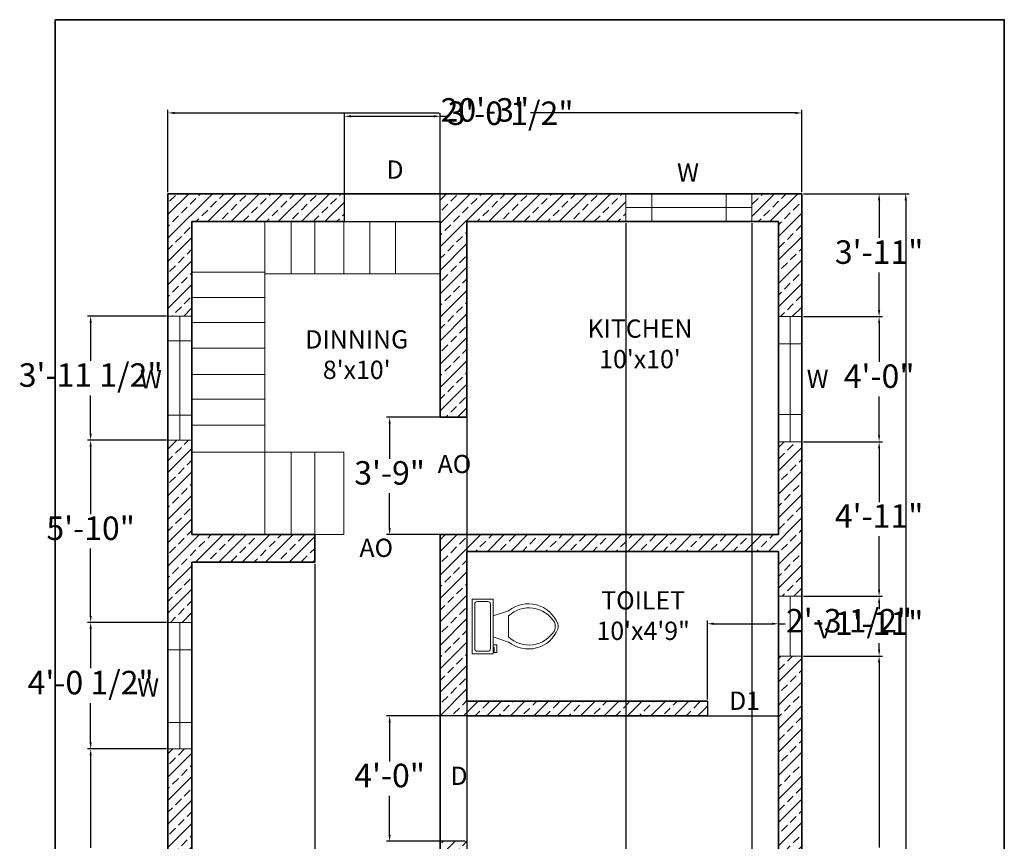
# Model space of a CAD drawing. Units: inches. Extents: x 3686 to 4476, y 4404 to 5066.
# Tile 2 of 2: x 3686 to 4064, y 4751 to 5066. Entities that reach past the tile are written whole.
import ezdxf

# ---------------------------------------------------------------- set-up
doc = ezdxf.new("R2010")
doc.units = ezdxf.units.IN
for name, color, linetype, lineweight in [('A-ANNO-DIMS', 3, 'Continuous', 18), ('A-ANNO-TEXT', 7, 'Continuous', 18), ('A-ANNO-TTLB', 7, 'Continuous', 35), ('A-AREA-IDEN', 7, 'Continuous', 25), ('A-DOOR', 3, 'Continuous', 25), ('A-FLOR-FIXT', 9, 'Continuous', 18), ('A-FLOR-STRS', 7, 'Continuous', 18), ('A-GLAZ', 4, 'Continuous', 18), ('A-WALL', 7, 'Continuous', 35), ('A-WALL-PATT', 8, 'Continuous', 13)]:
    doc.layers.add(name, color=color, linetype=linetype, lineweight=lineweight)
doc.styles.get("Standard").update_dxf_attribs({"font": 'arial.ttf'})
doc.dimstyles.new('ISO-25', dxfattribs={"dimtxt": 9, "dimasz": 2.5, "dimexe": 1.25, "dimexo": 0.625, "dimgap": 2, "dimtad": 0, "dimtih": 1, "dimtoh": 1, "dimdec": 1, "dimlunit": 4, "dimtxsty": 'Standard', "dimcen": 2.5, "dimadec": 0, "dimazin": 0, "dimtfac": 0.5, "dimtdec": 1, "dimtmove": 0, "dimatfit": 3, "dimfxl": 1, "dimarcsym": 0})

# ---------------------------------------------------------------- blocks, each defined once
blk = doc.blocks.new('*D1')
at = {"layer": 'A-ANNO-DIMS', "color": 0, "lineweight": -2, "transparency": 16777216}
for p, q in [((3743.02, 4999.94), (3743.02, 5031.48)), ((3745.52, 5030.23), (3846.98, 5030.23)), ((3983.52, 5030.23), (3882.05, 5030.23)), ((3986.02, 4999.94), (3986.02, 5031.48))]:
    blk.add_line(p, q, dxfattribs=at)
at = {"layer": 'A-ANNO-DIMS', "color": 0, "transparency": 16777216}
for points in [[(3745.52, 5030.65), (3745.52, 5029.82), (3743.02, 5030.23)], [(3983.52, 5030.65), (3983.52, 5029.82), (3986.02, 5030.23)]]:
    blk.add_solid(points, dxfattribs=at)
at = {"layer": 'Defpoints', "color": 0, "transparency": 16777216}
for p in [(3986.02, 5030.23), (3743.02, 4999.31), (3986.02, 4999.31)]:
    blk.add_point(p, dxfattribs=at)
at = {"layer": 'A-ANNO-DIMS', "color": 0, "transparency": 16777216, "insert": (3864.52, 5030.23), "char_height": 9, "attachment_point": 5}
blk.add_mtext('20\'-3"', dxfattribs=at)
blk = doc.blocks.new('*D2')
at = {"layer": 'A-ANNO-DIMS', "color": 0, "lineweight": -2, "transparency": 16777216}
for p, q in [((3986.64, 4999.31), (4027.13, 4999.31)), ((4025.88, 4996.81), (4025.88, 4729.91)), ((4025.88, 4449.81), (4025.88, 4716.72)), ((3986.64, 4447.31), (4027.13, 4447.31))]:
    blk.add_line(p, q, dxfattribs=at)
at = {"layer": 'A-ANNO-DIMS', "color": 0, "transparency": 16777216}
for points in [[(4025.46, 4996.81), (4026.3, 4996.81), (4025.88, 4999.31)], [(4025.46, 4449.81), (4026.3, 4449.81), (4025.88, 4447.31)]]:
    blk.add_solid(points, dxfattribs=at)
at = {"layer": 'Defpoints', "color": 0, "transparency": 16777216}
for p in [(3986.02, 4999.31), (3986.02, 4447.31), (4025.88, 4447.31)]:
    blk.add_point(p, dxfattribs=at)
at = {"layer": 'A-ANNO-DIMS', "color": 0, "transparency": 16777216, "insert": (4025.88, 4723.31), "char_height": 9, "attachment_point": 5}
blk.add_mtext("46'", dxfattribs=at)
blk = doc.blocks.new('*U6')
for p, q in [((9.5, -6), (9.5, -2)), ((-10, -8.5), (-8, -8.5)), ((-10, -9.5), (-10, -8.5)), ((-7, -9.5), (-10, -9.5)), ((-8, -8.5), (-8, -8)), ((-7, -8), (-7, -9.5)), ((-4, -8), (-6, -14)), ((4, -8), (6, -14)), ((4, -14), (-4, -14))]:
    blk.add_line(p, q)
blk.add_lwpolyline([(10.5, -8), (10.5, 0), (-10.5, 0), (-10.5, -8)], close=True)
for points in [[(-9.5, -2), (-9.5, -6)], [(8.5, -1), (-8.5, -1)], [(-8.5, -7), (8.5, -7)]]:
    blk.add_lwpolyline(points)
for centre, radius, start, end in [((-8.62, -1.88), 0.884, 81.8699, 188.1301), ((8.62, -1.88), 0.884, 351.8699, 98.1301), ((-8.62, -6.12), 0.884, 171.8699, 278.1301), ((8.62, -6.12), 0.884, 261.8699, 8.1301), ((3.52, -21.58), 12.17, 141.4691, 247.9714), ((4.2, -21.82), 11.33, 136.3677, 238.9468), ((-3.52, -21.58), 12.17, 292.0284, 38.5307), ((-4.2, -21.82), 11.33, 301.053, 43.6321), ((0, -27.88), 4, 245.7318, 294.2682), ((0, -29), 4, 254.8605, 285.1395)]:
    blk.add_arc(centre, radius, start, end)
blk = doc.blocks.new('*D13')
at = {"layer": 'A-ANNO-DIMS', "color": 0, "lineweight": -2, "transparency": 16777216}
for p, q in [((3810.64, 4989.22), (3810.64, 5030.21)), ((3813.14, 5028.96), (3844.89, 5028.96)), ((3847.39, 4989.22), (3847.39, 5030.21)), ((3847.39, 5028.96), (3849.89, 5028.96))]:
    blk.add_line(p, q, dxfattribs=at)
at = {"layer": 'A-ANNO-DIMS', "color": 0, "transparency": 16777216}
for points in [[(3813.14, 5029.38), (3813.14, 5028.55), (3810.64, 5028.96)], [(3844.89, 5029.38), (3844.89, 5028.55), (3847.39, 5028.96)]]:
    blk.add_solid(points, dxfattribs=at)
at = {"layer": 'Defpoints', "color": 0, "transparency": 16777216}
for p in [(3847.39, 5028.96), (3810.64, 4988.59), (3847.39, 4988.59)]:
    blk.add_point(p, dxfattribs=at)
at = {"layer": 'A-ANNO-DIMS', "color": 0, "transparency": 16777216, "insert": (3874.33, 5028.96), "char_height": 9, "attachment_point": 5}
blk.add_mtext('3\'-0 1/2"', dxfattribs=at)
blk = doc.blocks.new('*D14')
at = {"layer": 'A-ANNO-DIMS', "color": 0, "lineweight": -2, "transparency": 16777216}
for p, q in [((3857.64, 4987.97), (3857.64, 4416.41)), ((3918.61, 4987.97), (3918.61, 4416.41)), ((3860.14, 4417.66), (3874.16, 4417.66)), ((3916.11, 4417.66), (3902.09, 4417.66))]:
    blk.add_line(p, q, dxfattribs=at)
at = {"layer": 'A-ANNO-DIMS', "color": 0, "transparency": 16777216}
for points in [[(3860.14, 4418.08), (3860.14, 4417.25), (3857.64, 4417.66)], [(3916.11, 4418.08), (3916.11, 4417.25), (3918.61, 4417.66)]]:
    blk.add_solid(points, dxfattribs=at)
at = {"layer": 'Defpoints', "color": 0, "transparency": 16777216}
for p in [(3857.64, 4988.59), (3918.61, 4988.59), (3918.61, 4417.66)]:
    blk.add_point(p, dxfattribs=at)
at = {"layer": 'A-ANNO-DIMS', "color": 0, "transparency": 16777216, "insert": (3888.13, 4417.66), "char_height": 9, "attachment_point": 5}
blk.add_mtext('5\'-1"', dxfattribs=at)
blk = doc.blocks.new('*D15')
at = {"layer": 'A-ANNO-DIMS', "color": 0, "lineweight": -2, "transparency": 16777216}
for p, q in [((3918.61, 4987.97), (3918.61, 4416.41)), ((3966.81, 4987.97), (3966.81, 4416.41)), ((3921.11, 4417.66), (3928.57, 4417.66)), ((3964.31, 4417.66), (3956.85, 4417.66))]:
    blk.add_line(p, q, dxfattribs=at)
at = {"layer": 'A-ANNO-DIMS', "color": 0, "transparency": 16777216}
for points in [[(3921.11, 4418.08), (3921.11, 4417.25), (3918.61, 4417.66)], [(3964.31, 4418.08), (3964.31, 4417.25), (3966.81, 4417.66)]]:
    blk.add_solid(points, dxfattribs=at)
at = {"layer": 'Defpoints', "color": 0, "transparency": 16777216}
for p in [(3918.61, 4988.59), (3966.81, 4988.59), (3966.81, 4417.66)]:
    blk.add_point(p, dxfattribs=at)
at = {"layer": 'A-ANNO-DIMS', "color": 0, "transparency": 16777216, "insert": (3942.71, 4417.66), "char_height": 9, "attachment_point": 5}
blk.add_mtext('4\'-0"', dxfattribs=at)
blk = doc.blocks.new('*D16')
at = {"layer": 'A-ANNO-DIMS', "color": 0, "lineweight": -2, "transparency": 16777216}
for p, q in [((3986.64, 4999.31), (4016.92, 4999.31)), ((4015.67, 4996.81), (4015.67, 4982.36)), ((4015.67, 4954.71), (4015.67, 4969.16)), ((3986.64, 4952.21), (4016.92, 4952.21))]:
    blk.add_line(p, q, dxfattribs=at)
at = {"layer": 'A-ANNO-DIMS', "color": 0, "transparency": 16777216}
for points in [[(4015.25, 4996.81), (4016.08, 4996.81), (4015.67, 4999.31)], [(4015.25, 4954.71), (4016.08, 4954.71), (4015.67, 4952.21)]]:
    blk.add_solid(points, dxfattribs=at)
at = {"layer": 'Defpoints', "color": 0, "transparency": 16777216}
for p in [(3986.02, 4999.31), (3986.02, 4952.21), (4015.67, 4952.21)]:
    blk.add_point(p, dxfattribs=at)
at = {"layer": 'A-ANNO-DIMS', "color": 0, "transparency": 16777216, "insert": (4015.67, 4975.76), "char_height": 9, "attachment_point": 5}
blk.add_mtext('3\'-11"', dxfattribs=at)
blk = doc.blocks.new('*D17')
at = {"layer": 'A-ANNO-DIMS', "color": 0, "lineweight": -2, "transparency": 16777216}
for p, q in [((3986.64, 4952.21), (4016.92, 4952.21)), ((4015.67, 4949.71), (4015.67, 4934.82)), ((4015.67, 4906.73), (4015.67, 4921.63)), ((3986.64, 4904.23), (4016.92, 4904.23))]:
    blk.add_line(p, q, dxfattribs=at)
at = {"layer": 'A-ANNO-DIMS', "color": 0, "transparency": 16777216}
for points in [[(4015.25, 4949.71), (4016.08, 4949.71), (4015.67, 4952.21)], [(4015.25, 4906.73), (4016.08, 4906.73), (4015.67, 4904.23)]]:
    blk.add_solid(points, dxfattribs=at)
at = {"layer": 'Defpoints', "color": 0, "transparency": 16777216}
for p in [(3986.02, 4952.21), (3986.02, 4904.23), (4015.67, 4904.23)]:
    blk.add_point(p, dxfattribs=at)
at = {"layer": 'A-ANNO-DIMS', "color": 0, "transparency": 16777216, "insert": (4015.67, 4928.22), "char_height": 9, "attachment_point": 5}
blk.add_mtext('4\'-0"', dxfattribs=at)
blk = doc.blocks.new('*D18')
at = {"layer": 'A-ANNO-DIMS', "color": 0, "lineweight": -2, "transparency": 16777216}
for p, q in [((3986.64, 4904.23), (4016.92, 4904.23)), ((4015.67, 4901.73), (4015.67, 4881.17)), ((4015.67, 4847.58), (4015.67, 4868.14)), ((3986.64, 4845.08), (4016.92, 4845.08))]:
    blk.add_line(p, q, dxfattribs=at)
at = {"layer": 'A-ANNO-DIMS', "color": 0, "transparency": 16777216}
for points in [[(4015.25, 4901.73), (4016.08, 4901.73), (4015.67, 4904.23)], [(4015.25, 4847.58), (4016.08, 4847.58), (4015.67, 4845.08)]]:
    blk.add_solid(points, dxfattribs=at)
at = {"layer": 'Defpoints', "color": 0, "transparency": 16777216}
for p in [(3986.02, 4904.23), (3986.02, 4845.08), (4015.67, 4845.08)]:
    blk.add_point(p, dxfattribs=at)
at = {"layer": 'A-ANNO-DIMS', "color": 0, "transparency": 16777216, "insert": (4015.67, 4874.65), "char_height": 9, "attachment_point": 5}
blk.add_mtext('4\'-11"', dxfattribs=at)
blk = doc.blocks.new('*D19')
at = {"layer": 'A-ANNO-DIMS', "color": 0, "lineweight": -2, "transparency": 16777216}
for p, q in [((3986.64, 4845.08), (4016.92, 4845.08)), ((4015.67, 4842.58), (4015.67, 4840.11)), ((4015.67, 4824.62), (4015.67, 4827.08)), ((3986.64, 4822.12), (4016.92, 4822.12))]:
    blk.add_line(p, q, dxfattribs=at)
at = {"layer": 'A-ANNO-DIMS', "color": 0, "transparency": 16777216}
for points in [[(4015.25, 4842.58), (4016.08, 4842.58), (4015.67, 4845.08)], [(4015.25, 4824.62), (4016.08, 4824.62), (4015.67, 4822.12)]]:
    blk.add_solid(points, dxfattribs=at)
at = {"layer": 'Defpoints', "color": 0, "transparency": 16777216}
for p in [(3986.02, 4845.08), (3986.02, 4822.12), (4015.67, 4822.12)]:
    blk.add_point(p, dxfattribs=at)
at = {"layer": 'A-ANNO-DIMS', "color": 0, "transparency": 16777216, "insert": (4015.67, 4833.6), "char_height": 9, "attachment_point": 5}
blk.add_mtext('1\'-11"', dxfattribs=at)
blk = doc.blocks.new('*D20')
at = {"layer": 'A-ANNO-DIMS', "color": 0, "lineweight": -2, "transparency": 16777216}
for p, q in [((3986.64, 4822.12), (4016.92, 4822.12)), ((4015.67, 4819.62), (4015.67, 4748.74)), ((4015.67, 4664.68), (4015.67, 4735.55)), ((3986.64, 4662.18), (4016.92, 4662.18))]:
    blk.add_line(p, q, dxfattribs=at)
at = {"layer": 'A-ANNO-DIMS', "color": 0, "transparency": 16777216}
for points in [[(4015.25, 4819.62), (4016.08, 4819.62), (4015.67, 4822.12)], [(4015.25, 4664.68), (4016.08, 4664.68), (4015.67, 4662.18)]]:
    blk.add_solid(points, dxfattribs=at)
at = {"layer": 'Defpoints', "color": 0, "transparency": 16777216}
for p in [(3986.02, 4822.12), (3986.02, 4662.18), (4015.67, 4662.18)]:
    blk.add_point(p, dxfattribs=at)
at = {"layer": 'A-ANNO-DIMS', "color": 0, "transparency": 16777216, "insert": (4015.67, 4742.15), "char_height": 9, "attachment_point": 5}
blk.add_mtext('13\'-4"', dxfattribs=at)
blk = doc.blocks.new('*D22')
at = {"layer": 'A-ANNO-DIMS', "color": 0, "lineweight": -2, "transparency": 16777216}
for p, q in [((3742.39, 4952.43), (3712.12, 4952.43)), ((3713.37, 4949.93), (3713.37, 4935.3)), ((3713.37, 4907.37), (3713.37, 4921.99)), ((3742.39, 4904.87), (3712.12, 4904.87))]:
    blk.add_line(p, q, dxfattribs=at)
at = {"layer": 'A-ANNO-DIMS', "color": 0, "transparency": 16777216}
for points in [[(3712.95, 4949.93), (3713.78, 4949.93), (3713.37, 4952.43)], [(3712.95, 4907.37), (3713.78, 4907.37), (3713.37, 4904.87)]]:
    blk.add_solid(points, dxfattribs=at)
at = {"layer": 'Defpoints', "color": 0, "transparency": 16777216}
for p in [(3743.02, 4952.43), (3713.37, 4904.87), (3743.02, 4904.87)]:
    blk.add_point(p, dxfattribs=at)
at = {"layer": 'A-ANNO-DIMS', "color": 0, "transparency": 16777216, "insert": (3713.37, 4928.65), "char_height": 9, "attachment_point": 5}
blk.add_mtext('3\'-11 1/2"', dxfattribs=at)
blk = doc.blocks.new('*D23')
at = {"layer": 'A-ANNO-DIMS', "color": 0, "lineweight": -2, "transparency": 16777216}
for p, q in [((3742.39, 4904.87), (3712.12, 4904.87)), ((3713.37, 4902.37), (3713.37, 4876.55)), ((3713.37, 4837.55), (3713.37, 4863.36)), ((3742.39, 4835.05), (3712.12, 4835.05))]:
    blk.add_line(p, q, dxfattribs=at)
at = {"layer": 'A-ANNO-DIMS', "color": 0, "transparency": 16777216}
for points in [[(3712.95, 4902.37), (3713.78, 4902.37), (3713.37, 4904.87)], [(3712.95, 4837.55), (3713.78, 4837.55), (3713.37, 4835.05)]]:
    blk.add_solid(points, dxfattribs=at)
at = {"layer": 'Defpoints', "color": 0, "transparency": 16777216}
for p in [(3743.02, 4904.87), (3713.37, 4835.05), (3743.02, 4835.05)]:
    blk.add_point(p, dxfattribs=at)
at = {"layer": 'A-ANNO-DIMS', "color": 0, "transparency": 16777216, "insert": (3713.37, 4869.96), "char_height": 9, "attachment_point": 5}
blk.add_mtext('5\'-10"', dxfattribs=at)
blk = doc.blocks.new('*D24')
at = {"layer": 'A-ANNO-DIMS', "color": 0, "lineweight": -2, "transparency": 16777216}
for p, q in [((3742.39, 4835.05), (3712.12, 4835.05)), ((3713.37, 4832.55), (3713.37, 4817.47)), ((3713.37, 4789.08), (3713.37, 4804.16)), ((3742.39, 4786.58), (3712.12, 4786.58))]:
    blk.add_line(p, q, dxfattribs=at)
at = {"layer": 'A-ANNO-DIMS', "color": 0, "transparency": 16777216}
for points in [[(3712.95, 4832.55), (3713.78, 4832.55), (3713.37, 4835.05)], [(3712.95, 4789.08), (3713.78, 4789.08), (3713.37, 4786.58)]]:
    blk.add_solid(points, dxfattribs=at)
at = {"layer": 'Defpoints', "color": 0, "transparency": 16777216}
for p in [(3743.02, 4835.05), (3713.37, 4786.58), (3743.02, 4786.58)]:
    blk.add_point(p, dxfattribs=at)
at = {"layer": 'A-ANNO-DIMS', "color": 0, "transparency": 16777216, "insert": (3713.37, 4810.82), "char_height": 9, "attachment_point": 5}
blk.add_mtext('4\'-0 1/2"', dxfattribs=at)
blk = doc.blocks.new('*D25')
at = {"layer": 'A-ANNO-DIMS', "color": 0, "lineweight": -2, "transparency": 16777216}
for p, q in [((3742.39, 4786.58), (3712.12, 4786.58)), ((3713.37, 4784.08), (3713.37, 4748.64)), ((3713.37, 4700.05), (3713.37, 4735.49)), ((3742.39, 4697.55), (3712.12, 4697.55))]:
    blk.add_line(p, q, dxfattribs=at)
at = {"layer": 'A-ANNO-DIMS', "color": 0, "transparency": 16777216}
for points in [[(3712.95, 4784.08), (3713.78, 4784.08), (3713.37, 4786.58)], [(3712.95, 4700.05), (3713.78, 4700.05), (3713.37, 4697.55)]]:
    blk.add_solid(points, dxfattribs=at)
at = {"layer": 'Defpoints', "color": 0, "transparency": 16777216}
for p in [(3743.02, 4786.58), (3713.37, 4697.55), (3743.02, 4697.55)]:
    blk.add_point(p, dxfattribs=at)
at = {"layer": 'A-ANNO-DIMS', "color": 0, "transparency": 16777216, "insert": (3713.37, 4742.07), "char_height": 9, "attachment_point": 5}
blk.add_mtext('7\'-5"', dxfattribs=at)
blk = doc.blocks.new('*D33')
at = {"layer": 'A-ANNO-DIMS', "color": 0, "lineweight": -2, "transparency": 16777216}
for p, q in [((3857.02, 4799.25), (3826.74, 4799.25)), ((3827.99, 4796.75), (3827.99, 4781.81)), ((3827.99, 4753.67), (3827.99, 4768.62)), ((3857.02, 4751.17), (3826.74, 4751.17))]:
    blk.add_line(p, q, dxfattribs=at)
at = {"layer": 'A-ANNO-DIMS', "color": 0, "transparency": 16777216}
for points in [[(3827.58, 4796.75), (3828.41, 4796.75), (3827.99, 4799.25)], [(3827.58, 4753.67), (3828.41, 4753.67), (3827.99, 4751.17)]]:
    blk.add_solid(points, dxfattribs=at)
at = {"layer": 'Defpoints', "color": 0, "transparency": 16777216}
for p in [(3827.99, 4799.25), (3857.64, 4799.25), (3857.64, 4751.17)]:
    blk.add_point(p, dxfattribs=at)
at = {"layer": 'A-ANNO-DIMS', "color": 0, "transparency": 16777216, "insert": (3827.99, 4775.21), "char_height": 9, "attachment_point": 5}
blk.add_mtext('4\'-0"', dxfattribs=at)
blk = doc.blocks.new('*D34')
at = {"layer": 'A-ANNO-DIMS', "color": 0, "lineweight": -2, "transparency": 16777216}
for p, q in [((3949.83, 4805.48), (3949.83, 4835.76)), ((3952.33, 4834.51), (3974.61, 4834.51)), ((3977.11, 4805.48), (3977.11, 4835.76)), ((3977.11, 4834.51), (3979.61, 4834.51))]:
    blk.add_line(p, q, dxfattribs=at)
at = {"layer": 'A-ANNO-DIMS', "color": 0, "transparency": 16777216}
for points in [[(3952.33, 4834.93), (3952.33, 4834.09), (3949.83, 4834.51)], [(3974.61, 4834.93), (3974.61, 4834.09), (3977.11, 4834.51)]]:
    blk.add_solid(points, dxfattribs=at)
at = {"layer": 'Defpoints', "color": 0, "transparency": 16777216}
for p in [(3977.11, 4834.51), (3949.83, 4804.86), (3977.11, 4804.86)]:
    blk.add_point(p, dxfattribs=at)
at = {"layer": 'A-ANNO-DIMS', "color": 0, "transparency": 16777216, "insert": (4004.14, 4834.51), "char_height": 9, "attachment_point": 5}
blk.add_mtext('2\'-3 1/2"', dxfattribs=at)
blk = doc.blocks.new('*D35')
at = {"layer": 'A-ANNO-DIMS', "color": 0, "lineweight": -2, "transparency": 16777216}
for p, q in [((3799.26, 4857.46), (3799.26, 4416.41)), ((3847.39, 4857.46), (3847.39, 4416.41)), ((3801.76, 4417.66), (3809.18, 4417.66)), ((3844.89, 4417.66), (3837.47, 4417.66))]:
    blk.add_line(p, q, dxfattribs=at)
at = {"layer": 'A-ANNO-DIMS', "color": 0, "transparency": 16777216}
for points in [[(3801.76, 4418.08), (3801.76, 4417.25), (3799.26, 4417.66)], [(3844.89, 4418.08), (3844.89, 4417.25), (3847.39, 4417.66)]]:
    blk.add_solid(points, dxfattribs=at)
at = {"layer": 'Defpoints', "color": 0, "transparency": 16777216}
for p in [(3799.26, 4858.09), (3847.39, 4858.09), (3847.39, 4417.66)]:
    blk.add_point(p, dxfattribs=at)
at = {"layer": 'A-ANNO-DIMS', "color": 0, "transparency": 16777216, "insert": (3823.32, 4417.66), "char_height": 9, "attachment_point": 5}
blk.add_mtext('4\'-0"', dxfattribs=at)
blk = doc.blocks.new('*D36')
at = {"layer": 'A-ANNO-DIMS', "color": 0, "lineweight": -2, "transparency": 16777216}
for p, q in [((3857.02, 4913.66), (3826.74, 4913.66)), ((3827.99, 4911.16), (3827.99, 4897.77)), ((3827.99, 4871.19), (3827.99, 4884.58)), ((3857.02, 4868.69), (3826.74, 4868.69))]:
    blk.add_line(p, q, dxfattribs=at)
at = {"layer": 'A-ANNO-DIMS', "color": 0, "transparency": 16777216}
for points in [[(3827.58, 4911.16), (3828.41, 4911.16), (3827.99, 4913.66)], [(3827.58, 4871.19), (3828.41, 4871.19), (3827.99, 4868.69)]]:
    blk.add_solid(points, dxfattribs=at)
at = {"layer": 'Defpoints', "color": 0, "transparency": 16777216}
for p in [(3827.99, 4913.66), (3857.64, 4913.66), (3857.64, 4868.69)]:
    blk.add_point(p, dxfattribs=at)
at = {"layer": 'A-ANNO-DIMS', "color": 0, "transparency": 16777216, "insert": (3827.99, 4891.17), "char_height": 9, "attachment_point": 5}
blk.add_mtext('3\'-9"', dxfattribs=at)

msp = doc.modelspace()

# ---------------------------------------------------------------- hatches: boundary and pattern name
at = {"layer": 'A-WALL-PATT'}
h = msp.add_hatch(dxfattribs=at)
h.set_pattern_fill('ANSI33', color=256)
h.paths.add_polyline_path([(3810.64, 4999.31), (3743.02, 4999.31), (3743.02, 4952.43), (3752.2, 4952.43), (3752.2, 4988.59), (3810.64, 4988.59)])
h.paths.add_polyline_path([(3918.61, 4999.31), (3847.39, 4999.31), (3847.39, 4988.59), (3847.39, 4913.66), (3857.64, 4913.66), (3857.64, 4988.59), (3918.61, 4988.59)])
h.paths.add_polyline_path([(3986.02, 4999.31), (3966.81, 4999.31), (3966.81, 4988.59), (3977.11, 4988.59), (3977.11, 4952.21), (3986.02, 4952.21)])
h.paths.add_polyline_path([(3986.02, 4904.23), (3977.11, 4904.23), (3977.11, 4868.69), (3857.64, 4868.69), (3847.39, 4868.69), (3847.39, 4858.09), (3847.39, 4799.25), (3857.64, 4799.25), (3949.83, 4799.25), (3949.83, 4804.86), (3857.64, 4804.86), (3857.64, 4862.27), (3977.11, 4862.27), (3977.11, 4845.08), (3986.02, 4845.08)])
h.paths.add_polyline_path([(3986.02, 4822.12), (3977.11, 4822.12), (3977.11, 4662.18), (3986.02, 4662.18)])
h.paths.add_polyline_path([(3857.64, 4751.17), (3847.39, 4751.17), (3847.39, 4607.62), (3847.39, 4599.44), (3910.28, 4599.44), (3910.28, 4607.62), (3857.64, 4607.62)])
h.paths.add_polyline_path([(3986.02, 4614.69), (3977.11, 4614.69), (3977.11, 4607.62), (3957.66, 4607.62), (3957.66, 4599.44), (3986.02, 4599.44)])
h.paths.add_polyline_path([(3811.33, 4607.62), (3802.75, 4607.62), (3802.75, 4599.44), (3811.33, 4599.44)])
h.paths.add_polyline_path([(3752.2, 4649.55), (3743.02, 4649.55), (3743.02, 4599.44), (3754.88, 4599.44), (3754.88, 4607.62), (3752.2, 4607.62)])
h.paths.add_polyline_path([(3752.2, 4786.58), (3743.02, 4786.58), (3743.02, 4697.55), (3752.2, 4697.55)])
h.paths.add_polyline_path([(3799.26, 4868.69), (3752.2, 4868.69), (3752.2, 4904.87), (3743.02, 4904.87), (3743.02, 4835.05), (3752.2, 4835.05), (3752.2, 4858.09), (3799.26, 4858.09)])

# ---------------------------------------------------------------- linework, layer by layer
at = {"layer": 'A-ANNO-TTLB'}
msp.add_lwpolyline([(3699.7, 5065.96), (4063.67, 5065.96), (4063.67, 4404.9), (3699.7, 4404.9)], close=True, dxfattribs=at)
at = {"layer": 'A-DOOR'}
for p, q in [((3810.64, 4988.59), (3810.64, 4999.31)), ((3847.39, 4988.59), (3847.39, 4999.31)), ((3810.64, 4988.59), (3847.39, 4988.59)), ((3949.83, 4804.86), (3949.83, 4799.25)), ((3857.64, 4799.25), (3847.39, 4799.25)), ((3949.83, 4799.25), (3977.11, 4799.25))]:
    msp.add_line(p, q, dxfattribs=at)
at = {"layer": 'A-FLOR-STRS'}
for p, q in [((3780.14, 4868.69), (3780.14, 4988.59)), ((3790.28, 4968.57), (3790.28, 4988.59)), ((3799.26, 4968.57), (3799.26, 4988.59)), ((3810.43, 4968.57), (3810.43, 4988.59)), ((3820.43, 4968.57), (3820.43, 4988.59)), ((3830.24, 4968.57), (3830.24, 4988.59)), ((3780.14, 4969.25), (3752.2, 4969.25)), ((3847.39, 4968.57), (3780.14, 4968.57)), ((3780.14, 4968.57), (3780.14, 4900.33)), ((3780.14, 4959.58), (3752.2, 4959.58)), ((3780.14, 4949.92), (3752.2, 4949.92)), ((3780.14, 4940.1), (3752.2, 4940.1)), ((3780.14, 4930.02), (3752.2, 4930.02)), ((3780.14, 4920.56), (3752.2, 4920.56)), ((3780.14, 4910.62), (3752.2, 4910.62)), ((3780.14, 4900.33), (3752.2, 4900.33)), ((3780.14, 4900.33), (3810.43, 4900.33)), ((3790.28, 4868.69), (3790.28, 4900.33)), ((3799.26, 4868.69), (3799.26, 4900.33)), ((3810.43, 4868.69), (3810.43, 4900.33)), ((3799.26, 4868.69), (3810.43, 4868.69))]:
    msp.add_line(p, q, dxfattribs=at)
at = {"layer": 'A-GLAZ'}
for p, q in [((3918.61, 4999.31), (3918.61, 4988.59)), ((3928.57, 4999.31), (3928.57, 4988.59)), ((3957.08, 4999.31), (3957.08, 4988.59)), ((3966.81, 4999.31), (3966.81, 4988.59)), ((3966.81, 4993.95), (3918.61, 4993.95)), ((3752.2, 4952.43), (3743.02, 4952.43)), ((3747.61, 4952.43), (3747.61, 4904.87)), ((3977.11, 4952.21), (3986.02, 4952.21)), ((3981.56, 4952.21), (3981.56, 4904.23)), ((3752.2, 4942.95), (3743.02, 4942.95)), ((3977.11, 4941.78), (3986.02, 4941.78)), ((3752.2, 4914.43), (3743.02, 4914.43)), ((3977.11, 4914.66), (3986.02, 4914.66)), ((3752.2, 4904.87), (3743.02, 4904.87)), ((3977.11, 4904.23), (3986.02, 4904.23)), ((3977.11, 4845.08), (3986.02, 4845.08)), ((3981.56, 4845.08), (3981.56, 4822.12)), ((3743.02, 4835.05), (3752.2, 4835.05)), ((3747.61, 4835.05), (3747.61, 4786.58)), ((3743.02, 4824.57), (3752.2, 4824.57)), ((3977.11, 4822.12), (3986.02, 4822.12)), ((3743.02, 4796.64), (3752.2, 4796.64)), ((3743.02, 4786.58), (3752.2, 4786.58))]:
    msp.add_line(p, q, dxfattribs=at)
at = {"layer": 'A-WALL'}
for p, q in [((3743.02, 4999.31), (3986.02, 4999.31)), ((3743.02, 4447.31), (3743.02, 4999.31)), ((3986.02, 4599.44), (3986.02, 4999.31)), ((3752.2, 4988.59), (3810.64, 4988.59)), ((3752.2, 4868.69), (3752.2, 4988.59)), ((3847.39, 4913.66), (3847.39, 4988.59)), ((3857.64, 4988.59), (3977.11, 4988.59)), ((3857.64, 4913.66), (3857.64, 4988.59)), ((3977.11, 4988.59), (3977.11, 4868.69)), ((3857.64, 4913.66), (3847.39, 4913.66)), ((3752.2, 4868.69), (3799.26, 4868.69)), ((3799.26, 4868.69), (3799.26, 4858.09)), ((3847.39, 4868.69), (3847.39, 4858.09)), ((3857.64, 4868.69), (3847.39, 4868.69)), ((3857.64, 4868.69), (3977.11, 4868.69)), ((3857.64, 4862.27), (3977.11, 4862.27)), ((3857.64, 4804.86), (3857.64, 4862.27)), ((3977.11, 4862.27), (3977.11, 4804.86)), ((3977.11, 4862.27), (3977.11, 4607.62)), ((3752.2, 4858.09), (3799.26, 4858.09)), ((3752.2, 4607.62), (3752.2, 4858.09)), ((3847.39, 4607.62), (3847.39, 4858.09)), ((3857.64, 4804.86), (3949.83, 4804.86)), ((3857.64, 4799.25), (3949.83, 4799.25))]:
    msp.add_line(p, q, dxfattribs=at)

# ---------------------------------------------------------------- block references
at = {"layer": 'A-FLOR-FIXT', "rotation": 90}
msp.add_blockref('*U6', (3859.63, 4833.5), dxfattribs=at)

# ---------------------------------------------------------------- texts
at = {"layer": 'A-ANNO-TEXT', "char_height": 7, "attachment_point": 1}
for s, width, insert in [('\\pxqc;{\\fArial|b1|i0|c0|p34;D}', 21.499, (3819.31, 5012.02)), ('\\pxqc;{\\fArial|b1|i0|c0|p34;W}', 21.499, (3931.64, 5010.87)), ('\\pxqc;{\\fArial|b1|i0|c0|p34;W}', 21.499, (3725.71, 4931.7)), ('\\pxqc;{\\fArial|b1|i0|c0|p34;W}', 21.499, (3981.34, 4931.88)), ('\\pxqc;{\\fArial|b1|i0|c0|p34;AO}', 19.1815, (3843.24, 4899.23)), ('\\pxqc;{\\fArial|b1|i0|c0|p34;AO}', 19.1815, (3813.27, 4867.12)), ('\\pxqc;{\\fArial|b1|i0|c0|p34;V}', 21.499, (3983.93, 4835.9)), ('\\pxqc;{\\fArial|b1|i0|c0|p34;W}', 21.499, (3724.64, 4813.58)), ('\\pxqc;{\\fArial|b1|i0|c0|p34;D1}', 21.499, (3953.35, 4808.54)), ('\\pxqc;{\\fArial|b1|i0|c0|p34;D}', 21.499, (3843.87, 4779.76))]:
    msp.add_mtext_dynamic_manual_height_columns(s, width=width, gutter_width=12.5, heights=[0], dxfattribs=dict(at, insert=insert))
at = {"layer": 'A-AREA-IDEN', "char_height": 7, "attachment_point": 1}
for s, width, insert in [("\\pxqc;{\\fArial|b1|i0|c0|p34;KITCHEN\\P10'x10'}", 79.6112, (3884.18, 4951.1)), ("\\pxqc;{\\fArial|b1|i0|c0|p34;DINNING\\P8'x10'}", 57.609, (3786.57, 4946.98)), ('\\pxqc;{\\fArial|b1|i0|c0|p34;TOILET\\P10\'x4\'9"}', 74.291, (3888.06, 4846.99))]:
    msp.add_mtext_dynamic_manual_height_columns(s, width=width, gutter_width=12.5, heights=[0], dxfattribs=dict(at, insert=insert))

# ---------------------------------------------------------------- dimensions: what is measured, and where the dimension line sits
at = {"layer": 'A-ANNO-DIMS'}
for base, p1, p2, override, picture, middle in [((3847.3851, 5028.9637), (3810.6399, 4988.5907), (3847.3851, 4988.5907), {"dimdec": 1, "dimlfac": 1, "dimrnd": 0, "dimzin": 1, "dimdsep": 46, "dimlunit": 4, "dimfrac": 2}, '*D13', (3874.3299, 5028.9637)), ((3986.02, 5030.23), (3743.02, 4999.31), (3986.02, 4999.31), {"dimclrd": 0, "dimclre": 0, "dimclrt": 0}, '*D1', (3864.52, 5030.23)), ((3918.61, 4417.66), (3857.64, 4988.59), (3918.61, 4988.59), {"dimdec": 1, "dimlfac": 1, "dimrnd": 0, "dimzin": 1, "dimdsep": 46, "dimlunit": 4, "dimfrac": 2}, '*D14', (3888.13, 4417.66)), ((3966.81, 4417.66), (3918.61, 4988.59), (3966.81, 4988.59), {"dimdec": 1, "dimlfac": 1, "dimrnd": 0, "dimzin": 1, "dimdsep": 46, "dimlunit": 4, "dimfrac": 2}, '*D15', (3942.71, 4417.66)), ((3847.39, 4417.66), (3799.26, 4858.09), (3847.39, 4858.09), {"dimdec": 1, "dimlfac": 1, "dimrnd": 0, "dimzin": 1, "dimdsep": 46, "dimlunit": 4, "dimfrac": 2}, '*D35', (3823.32, 4417.66)), ((3977.11, 4834.51), (3949.83, 4804.86), (3977.11, 4804.86), {"dimdec": 1, "dimlfac": 1, "dimrnd": 0, "dimzin": 1, "dimdsep": 46, "dimlunit": 4, "dimfrac": 2}, '*D34', (4004.14, 4834.51))]:
    dim = msp.add_linear_dim(base=base, p1=p1, p2=p2, dimstyle='ISO-25', override=override, dxfattribs=at)
    dim.commit()
    dim.dimension.update_dxf_attribs({"geometry": picture, "text_midpoint": middle})
for base, p1, p2, override, picture, middle in [((4025.88, 4447.31), (3986.02, 4999.31), (3986.02, 4447.31), {"dimclrd": 0, "dimclre": 0, "dimclrt": 0}, '*D2', (4025.88, 4723.31)), ((4015.67, 4952.21), (3986.02, 4999.31), (3986.02, 4952.21), {"dimdec": 1, "dimlfac": 1, "dimrnd": 0, "dimzin": 1, "dimdsep": 46, "dimlunit": 4, "dimfrac": 2}, '*D16', (4015.67, 4975.76)), ((3713.37, 4904.87), (3743.02, 4952.43), (3743.02, 4904.87), {"dimdec": 1, "dimlfac": 1, "dimrnd": 0, "dimzin": 1, "dimdsep": 46, "dimlunit": 4, "dimfrac": 2}, '*D22', (3713.37, 4928.65)), ((4015.67, 4904.23), (3986.02, 4952.21), (3986.02, 4904.23), {"dimdec": 1, "dimlfac": 1, "dimrnd": 0, "dimzin": 1, "dimdsep": 46, "dimlunit": 4, "dimfrac": 2}, '*D17', (4015.67, 4928.22)), ((3827.99, 4913.66), (3857.64, 4868.69), (3857.64, 4913.66), {"dimdec": 1, "dimlfac": 1, "dimrnd": 0, "dimzin": 1, "dimdsep": 46, "dimlunit": 4, "dimfrac": 2}, '*D36', (3827.99, 4891.17)), ((3713.37, 4835.05), (3743.02, 4904.87), (3743.02, 4835.05), {"dimdec": 1, "dimlfac": 1, "dimrnd": 0, "dimzin": 1, "dimdsep": 46, "dimlunit": 4, "dimfrac": 2}, '*D23', (3713.37, 4869.96)), ((4015.6683, 4845.0763), (3986.0183, 4904.2308), (3986.0183, 4845.0763), {"dimdec": 1, "dimlfac": 1, "dimrnd": 0, "dimzin": 1, "dimdsep": 46, "dimlunit": 4, "dimfrac": 2}, '*D18', (4015.6683, 4874.6536)), ((4015.67, 4822.12), (3986.02, 4845.08), (3986.02, 4822.12), {"dimdec": 1, "dimlfac": 1, "dimrnd": 0, "dimzin": 1, "dimdsep": 46, "dimlunit": 4, "dimfrac": 2}, '*D19', (4015.67, 4833.6)), ((3713.37, 4786.58), (3743.02, 4835.05), (3743.02, 4786.58), {"dimdec": 1, "dimlfac": 1, "dimrnd": 0, "dimzin": 1, "dimdsep": 46, "dimlunit": 4, "dimfrac": 2}, '*D24', (3713.37, 4810.82)), ((4015.67, 4662.18), (3986.02, 4822.12), (3986.02, 4662.18), {"dimdec": 1, "dimlfac": 1, "dimrnd": 0, "dimzin": 1, "dimdsep": 46, "dimlunit": 4, "dimfrac": 2}, '*D20', (4015.67, 4742.15)), ((3827.99, 4799.25), (3857.64, 4751.17), (3857.64, 4799.25), {"dimdec": 1, "dimlfac": 1, "dimrnd": 0, "dimzin": 1, "dimdsep": 46, "dimlunit": 4, "dimfrac": 2}, '*D33', (3827.99, 4775.21)), ((3713.37, 4697.55), (3743.02, 4786.58), (3743.02, 4697.55), {"dimdec": 1, "dimlfac": 1, "dimrnd": 0, "dimzin": 1, "dimdsep": 46, "dimlunit": 4, "dimfrac": 2}, '*D25', (3713.37, 4742.07))]:
    dim = msp.add_linear_dim(base=base, p1=p1, p2=p2, angle=90, dimstyle='ISO-25', override=override, dxfattribs=at)
    dim.commit()
    dim.dimension.update_dxf_attribs({"geometry": picture, "text_midpoint": middle})

doc.saveas('drawing.dxf')
